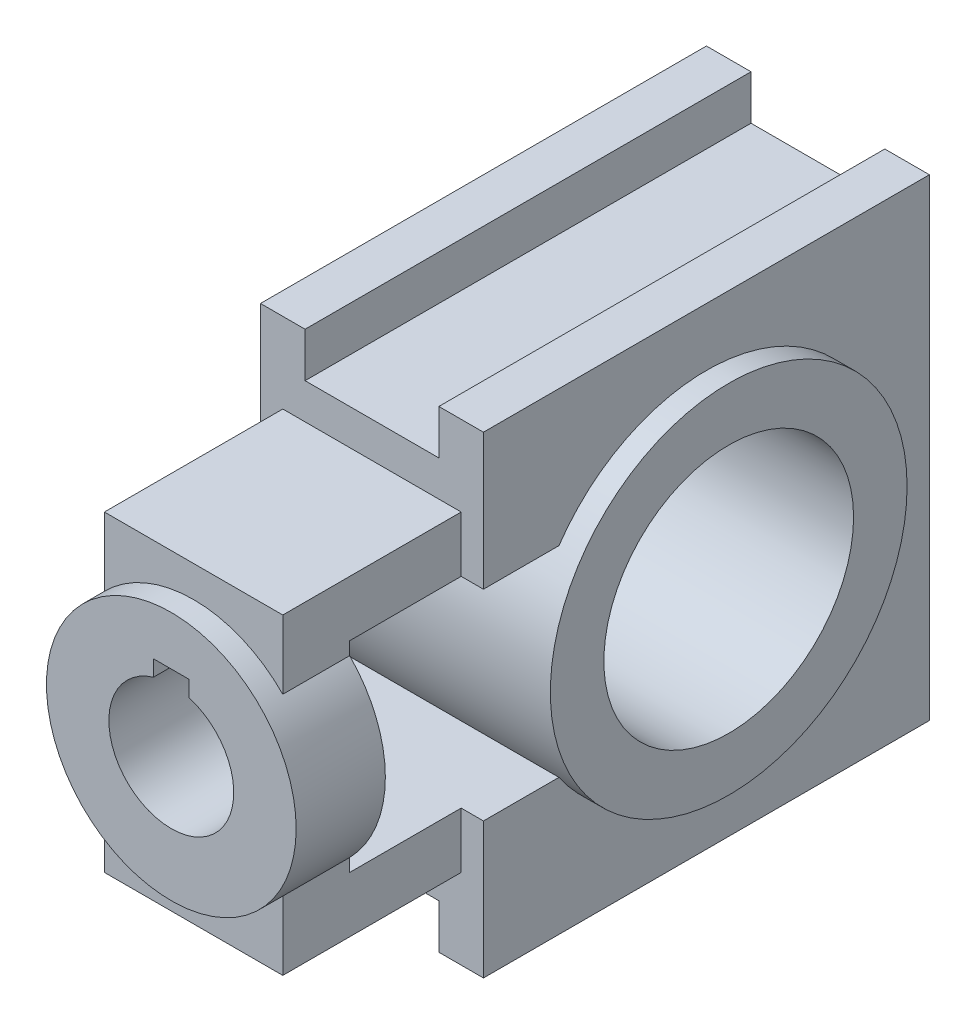
ISO-10303-21;
HEADER;
FILE_DESCRIPTION(('STEP AP214'),'2;1');
FILE_NAME('part.step','',(''),(''),'','','');
FILE_SCHEMA(('AUTOMOTIVE_DESIGN { 1 0 10303 214 1 1 1 1 }'));
ENDSEC;
DATA;
#1=APPLICATION_CONTEXT('core data for automotive mechanical design processes');
#2=APPLICATION_PROTOCOL_DEFINITION('international standard','automotive_design',2000,#1);
#3=PRODUCT_CONTEXT('',#1,'mechanical');
#4=PRODUCT('Part','Part','',(#3));
#5=PRODUCT_RELATED_PRODUCT_CATEGORY('part','',(#4));
#6=PRODUCT_DEFINITION_FORMATION('','',#4);
#7=PRODUCT_DEFINITION_CONTEXT('part definition',#1,'design');
#8=PRODUCT_DEFINITION('design','',#6,#7);
#9=PRODUCT_DEFINITION_SHAPE('','',#8);
#10=(LENGTH_UNIT() NAMED_UNIT(*) SI_UNIT(.MILLI.,.METRE.));
#11=(NAMED_UNIT(*) PLANE_ANGLE_UNIT() SI_UNIT($,.RADIAN.));
#12=(NAMED_UNIT(*) SI_UNIT($,.STERADIAN.) SOLID_ANGLE_UNIT());
#13=UNCERTAINTY_MEASURE_WITH_UNIT(LENGTH_MEASURE(1.E-05),#10,'distance_accuracy_value','');
#14=(GEOMETRIC_REPRESENTATION_CONTEXT(3) GLOBAL_UNCERTAINTY_ASSIGNED_CONTEXT((#13)) GLOBAL_UNIT_ASSIGNED_CONTEXT((#10,
#11,#12)) REPRESENTATION_CONTEXT('',''));
#15=CARTESIAN_POINT('',(0.,0.,0.));
#16=DIRECTION('',(0.,0.,1.));
#17=DIRECTION('',(1.,0.,0.));
#18=AXIS2_PLACEMENT_3D('',#15,#16,#17);
#19=CARTESIAN_POINT('',(-50.,-53.,50.));
#20=DIRECTION('',(0.,-1.,0.));
#21=DIRECTION('',(0.,0.,-1.));
#22=AXIS2_PLACEMENT_3D('',#19,#20,#21);
#23=PLANE('',#22);
#24=DIRECTION('',(0.,0.,1.));
#25=VECTOR('',#24,1.);
#26=CARTESIAN_POINT('',(-10.,-53.,-50.));
#27=LINE('',#26,#25);
#28=CARTESIAN_POINT('',(-10.,-53.,-50.));
#29=VERTEX_POINT('',#28);
#30=CARTESIAN_POINT('',(-10.,-53.,50.));
#31=VERTEX_POINT('',#30);
#32=EDGE_CURVE('E261',#29,#31,#27,.T.);
#33=ORIENTED_EDGE('',*,*,#32,.F.);
#34=DIRECTION('',(1.,0.,0.));
#35=VECTOR('',#34,1.);
#36=CARTESIAN_POINT('',(-50.,-53.,-50.));
#37=LINE('',#36,#35);
#38=CARTESIAN_POINT('',(0.,-53.,-50.));
#39=VERTEX_POINT('',#38);
#40=EDGE_CURVE('E475',#29,#39,#37,.T.);
#41=ORIENTED_EDGE('',*,*,#40,.T.);
#42=DIRECTION('',(0.,0.,-1.));
#43=VECTOR('',#42,1.);
#44=CARTESIAN_POINT('',(0.,-53.,50.));
#45=LINE('',#44,#43);
#46=CARTESIAN_POINT('',(0.,-53.,50.));
#47=VERTEX_POINT('',#46);
#48=EDGE_CURVE('E448',#47,#39,#45,.T.);
#49=ORIENTED_EDGE('',*,*,#48,.F.);
#50=DIRECTION('',(1.,0.,0.));
#51=VECTOR('',#50,1.);
#52=CARTESIAN_POINT('',(-50.,-53.,50.));
#53=LINE('',#52,#51);
#54=EDGE_CURVE('E479',#31,#47,#53,.T.);
#55=ORIENTED_EDGE('',*,*,#54,.F.);
#56=EDGE_LOOP('',(#33,#41,#49,#55));
#57=FACE_BOUND('',#56,.T.);
#58=ADVANCED_FACE('F39',(#57),#23,.T.);
#59=CARTESIAN_POINT('',(-50.,0.,0.));
#60=DIRECTION('',(1.,0.,0.));
#61=DIRECTION('',(0.,0.,-1.));
#62=AXIS2_PLACEMENT_3D('',#59,#60,#61);
#63=PLANE('',#62);
#64=CARTESIAN_POINT('',(-50.,0.,0.));
#65=DIRECTION('',(-1.,0.,0.));
#66=DIRECTION('',(0.,0.,1.));
#67=AXIS2_PLACEMENT_3D('',#64,#65,#66);
#68=CIRCLE('',#67,40.);
#69=CARTESIAN_POINT('',(-50.,22.5,33.0718913883074));
#70=VERTEX_POINT('',#69);
#71=CARTESIAN_POINT('',(-50.,-22.5,33.0718913883074));
#72=VERTEX_POINT('',#71);
#73=EDGE_CURVE('E279',#70,#72,#68,.T.);
#74=ORIENTED_EDGE('',*,*,#73,.F.);
#75=DIRECTION('',(0.,0.,1.));
#76=VECTOR('',#75,1.);
#77=CARTESIAN_POINT('',(-50.,22.5,50.));
#78=LINE('',#77,#76);
#79=CARTESIAN_POINT('',(-50.,22.5,50.));
#80=VERTEX_POINT('',#79);
#81=EDGE_CURVE('E424',#70,#80,#78,.T.);
#82=ORIENTED_EDGE('',*,*,#81,.T.);
#83=DIRECTION('',(0.,-1.,0.));
#84=VECTOR('',#83,1.);
#85=CARTESIAN_POINT('',(-50.,53.,50.));
#86=LINE('',#85,#84);
#87=CARTESIAN_POINT('',(-50.,53.,50.));
#88=VERTEX_POINT('',#87);
#89=EDGE_CURVE('E455',#88,#80,#86,.T.);
#90=ORIENTED_EDGE('',*,*,#89,.F.);
#91=DIRECTION('',(0.,0.,1.));
#92=VECTOR('',#91,1.);
#93=CARTESIAN_POINT('',(-50.,53.,-50.));
#94=LINE('',#93,#92);
#95=CARTESIAN_POINT('',(-50.,53.,-50.));
#96=VERTEX_POINT('',#95);
#97=EDGE_CURVE('E446',#96,#88,#94,.T.);
#98=ORIENTED_EDGE('',*,*,#97,.F.);
#99=DIRECTION('',(0.,1.,0.));
#100=VECTOR('',#99,1.);
#101=CARTESIAN_POINT('',(-50.,-53.,-50.));
#102=LINE('',#101,#100);
#103=CARTESIAN_POINT('',(-50.,-53.,-50.));
#104=VERTEX_POINT('',#103);
#105=EDGE_CURVE('E450',#104,#96,#102,.T.);
#106=ORIENTED_EDGE('',*,*,#105,.F.);
#107=DIRECTION('',(0.,0.,-1.));
#108=VECTOR('',#107,1.);
#109=CARTESIAN_POINT('',(-50.,-53.,50.));
#110=LINE('',#109,#108);
#111=CARTESIAN_POINT('',(-50.,-53.,50.));
#112=VERTEX_POINT('',#111);
#113=EDGE_CURVE('E456',#112,#104,#110,.T.);
#114=ORIENTED_EDGE('',*,*,#113,.F.);
#115=CARTESIAN_POINT('',(-50.,-22.5,50.));
#116=VERTEX_POINT('',#115);
#117=EDGE_CURVE('E452',#116,#112,#86,.T.);
#118=ORIENTED_EDGE('',*,*,#117,.F.);
#119=DIRECTION('',(0.,0.,-1.));
#120=VECTOR('',#119,1.);
#121=CARTESIAN_POINT('',(-50.,-22.5,50.));
#122=LINE('',#121,#120);
#123=EDGE_CURVE('E422',#116,#72,#122,.T.);
#124=ORIENTED_EDGE('',*,*,#123,.T.);
#125=EDGE_LOOP('',(#74,#82,#90,#98,#106,#114,#118,#124));
#126=FACE_BOUND('',#125,.T.);
#127=ADVANCED_FACE('F539',(#126),#63,.F.);
#128=CARTESIAN_POINT('',(-45.,0.,90.));
#129=DIRECTION('',(0.,0.,1.));
#130=DIRECTION('',(1.,0.,0.));
#131=AXIS2_PLACEMENT_3D('',#128,#129,#130);
#132=PLANE('',#131);
#133=CARTESIAN_POINT('',(-25.,0.,90.));
#134=DIRECTION('',(0.,0.,1.));
#135=DIRECTION('',(1.,0.,0.));
#136=AXIS2_PLACEMENT_3D('',#133,#134,#135);
#137=CIRCLE('',#136,28.);
#138=CARTESIAN_POINT('',(-5.,19.5959179422654,90.));
#139=VERTEX_POINT('',#138);
#140=CARTESIAN_POINT('',(-45.,19.5959179422654,90.));
#141=VERTEX_POINT('',#140);
#142=EDGE_CURVE('E314',#139,#141,#137,.T.);
#143=ORIENTED_EDGE('',*,*,#142,.F.);
#144=DIRECTION('',(0.,-1.,0.));
#145=VECTOR('',#144,1.);
#146=CARTESIAN_POINT('',(-5.,0.,90.));
#147=LINE('',#146,#145);
#148=CARTESIAN_POINT('',(-5.,35.,90.));
#149=VERTEX_POINT('',#148);
#150=EDGE_CURVE('E370',#149,#139,#147,.T.);
#151=ORIENTED_EDGE('',*,*,#150,.F.);
#152=DIRECTION('',(1.,0.,0.));
#153=VECTOR('',#152,1.);
#154=CARTESIAN_POINT('',(-45.,35.,90.));
#155=LINE('',#154,#153);
#156=CARTESIAN_POINT('',(-45.,35.,90.));
#157=VERTEX_POINT('',#156);
#158=EDGE_CURVE('E379',#157,#149,#155,.T.);
#159=ORIENTED_EDGE('',*,*,#158,.F.);
#160=DIRECTION('',(0.,-1.,0.));
#161=VECTOR('',#160,1.);
#162=CARTESIAN_POINT('',(-45.,0.,90.));
#163=LINE('',#162,#161);
#164=EDGE_CURVE('E344',#157,#141,#163,.T.);
#165=ORIENTED_EDGE('',*,*,#164,.T.);
#166=EDGE_LOOP('',(#143,#151,#159,#165));
#167=FACE_BOUND('',#166,.T.);
#168=ADVANCED_FACE('F560',(#167),#132,.T.);
#169=CARTESIAN_POINT('',(-45.,0.,0.));
#170=DIRECTION('',(1.,0.,0.));
#171=DIRECTION('',(0.,0.,-1.));
#172=AXIS2_PLACEMENT_3D('',#169,#170,#171);
#173=PLANE('',#172);
#174=DIRECTION('',(0.,1.,0.));
#175=VECTOR('',#174,1.);
#176=CARTESIAN_POINT('',(-45.,22.5,75.));
#177=LINE('',#176,#175);
#178=CARTESIAN_POINT('',(-45.,19.5959179422654,75.));
#179=VERTEX_POINT('',#178);
#180=CARTESIAN_POINT('',(-45.,22.5,75.));
#181=VERTEX_POINT('',#180);
#182=EDGE_CURVE('E330',#179,#181,#177,.T.);
#183=ORIENTED_EDGE('',*,*,#182,.F.);
#184=DIRECTION('',(0.,0.,1.));
#185=VECTOR('',#184,1.);
#186=CARTESIAN_POINT('',(-45.,19.5959179422654,75.));
#187=LINE('',#186,#185);
#188=EDGE_CURVE('E323',#179,#141,#187,.T.);
#189=ORIENTED_EDGE('',*,*,#188,.T.);
#190=ORIENTED_EDGE('',*,*,#164,.F.);
#191=DIRECTION('',(0.,0.,1.));
#192=VECTOR('',#191,1.);
#193=CARTESIAN_POINT('',(-45.,35.,90.));
#194=LINE('',#193,#192);
#195=CARTESIAN_POINT('',(-45.,35.,50.));
#196=VERTEX_POINT('',#195);
#197=EDGE_CURVE('E336',#196,#157,#194,.T.);
#198=ORIENTED_EDGE('',*,*,#197,.F.);
#199=DIRECTION('',(0.,1.,0.));
#200=VECTOR('',#199,1.);
#201=CARTESIAN_POINT('',(-45.,35.,50.));
#202=LINE('',#201,#200);
#203=CARTESIAN_POINT('',(-45.,22.5,50.));
#204=VERTEX_POINT('',#203);
#205=EDGE_CURVE('E337',#204,#196,#202,.T.);
#206=ORIENTED_EDGE('',*,*,#205,.F.);
#207=DIRECTION('',(0.,0.,-1.));
#208=VECTOR('',#207,1.);
#209=CARTESIAN_POINT('',(-45.,22.5,50.));
#210=LINE('',#209,#208);
#211=EDGE_CURVE('E333',#181,#204,#210,.T.);
#212=ORIENTED_EDGE('',*,*,#211,.F.);
#213=EDGE_LOOP('',(#183,#189,#190,#198,#206,#212));
#214=FACE_BOUND('',#213,.T.);
#215=ADVANCED_FACE('F550',(#214),#173,.F.);
#216=CARTESIAN_POINT('',(-5.,0.,0.));
#217=DIRECTION('',(1.,0.,0.));
#218=DIRECTION('',(0.,0.,-1.));
#219=AXIS2_PLACEMENT_3D('',#216,#217,#218);
#220=PLANE('',#219);
#221=DIRECTION('',(0.,0.,1.));
#222=VECTOR('',#221,1.);
#223=CARTESIAN_POINT('',(-5.,19.5959179422654,75.));
#224=LINE('',#223,#222);
#225=CARTESIAN_POINT('',(-5.,19.5959179422654,75.));
#226=VERTEX_POINT('',#225);
#227=EDGE_CURVE('E11',#226,#139,#224,.T.);
#228=ORIENTED_EDGE('',*,*,#227,.F.);
#229=DIRECTION('',(0.,1.,0.));
#230=VECTOR('',#229,1.);
#231=CARTESIAN_POINT('',(-5.,22.5,75.));
#232=LINE('',#231,#230);
#233=CARTESIAN_POINT('',(-5.,22.5,75.));
#234=VERTEX_POINT('',#233);
#235=EDGE_CURVE('E353',#226,#234,#232,.T.);
#236=ORIENTED_EDGE('',*,*,#235,.T.);
#237=DIRECTION('',(0.,0.,-1.));
#238=VECTOR('',#237,1.);
#239=CARTESIAN_POINT('',(-5.,22.5,50.));
#240=LINE('',#239,#238);
#241=CARTESIAN_POINT('',(-5.,22.5,50.));
#242=VERTEX_POINT('',#241);
#243=EDGE_CURVE('E357',#234,#242,#240,.T.);
#244=ORIENTED_EDGE('',*,*,#243,.T.);
#245=DIRECTION('',(0.,1.,0.));
#246=VECTOR('',#245,1.);
#247=CARTESIAN_POINT('',(-5.,35.,50.));
#248=LINE('',#247,#246);
#249=CARTESIAN_POINT('',(-5.,35.,50.));
#250=VERTEX_POINT('',#249);
#251=EDGE_CURVE('E359',#242,#250,#248,.T.);
#252=ORIENTED_EDGE('',*,*,#251,.T.);
#253=DIRECTION('',(0.,0.,1.));
#254=VECTOR('',#253,1.);
#255=CARTESIAN_POINT('',(-5.,35.,90.));
#256=LINE('',#255,#254);
#257=EDGE_CURVE('E361',#250,#149,#256,.T.);
#258=ORIENTED_EDGE('',*,*,#257,.T.);
#259=ORIENTED_EDGE('',*,*,#150,.T.);
#260=EDGE_LOOP('',(#228,#236,#244,#252,#258,#259));
#261=FACE_BOUND('',#260,.T.);
#262=ADVANCED_FACE('F551',(#261),#220,.T.);
#263=CARTESIAN_POINT('',(-50.,53.,50.));
#264=DIRECTION('',(0.,0.,1.));
#265=DIRECTION('',(0.,-1.,0.));
#266=AXIS2_PLACEMENT_3D('',#263,#264,#265);
#267=PLANE('',#266);
#268=DIRECTION('',(1.,0.,0.));
#269=VECTOR('',#268,1.);
#270=CARTESIAN_POINT('',(-50.,22.5,50.));
#271=LINE('',#270,#269);
#272=EDGE_CURVE('E432',#80,#204,#271,.T.);
#273=ORIENTED_EDGE('',*,*,#272,.T.);
#274=ORIENTED_EDGE('',*,*,#205,.T.);
#275=DIRECTION('',(1.,0.,0.));
#276=VECTOR('',#275,1.);
#277=CARTESIAN_POINT('',(-45.,35.,50.));
#278=LINE('',#277,#276);
#279=EDGE_CURVE('E384',#196,#250,#278,.T.);
#280=ORIENTED_EDGE('',*,*,#279,.T.);
#281=ORIENTED_EDGE('',*,*,#251,.F.);
#282=CARTESIAN_POINT('',(0.,22.5,50.));
#283=VERTEX_POINT('',#282);
#284=EDGE_CURVE('E440',#242,#283,#271,.T.);
#285=ORIENTED_EDGE('',*,*,#284,.T.);
#286=DIRECTION('',(0.,-1.,0.));
#287=VECTOR('',#286,1.);
#288=CARTESIAN_POINT('',(0.,53.,50.));
#289=LINE('',#288,#287);
#290=CARTESIAN_POINT('',(0.,53.,50.));
#291=VERTEX_POINT('',#290);
#292=EDGE_CURVE('E470',#291,#283,#289,.T.);
#293=ORIENTED_EDGE('',*,*,#292,.F.);
#294=DIRECTION('',(1.,0.,0.));
#295=VECTOR('',#294,1.);
#296=CARTESIAN_POINT('',(-50.,53.,50.));
#297=LINE('',#296,#295);
#298=CARTESIAN_POINT('',(-10.,53.,50.));
#299=VERTEX_POINT('',#298);
#300=EDGE_CURVE('E477',#299,#291,#297,.T.);
#301=ORIENTED_EDGE('',*,*,#300,.F.);
#302=DIRECTION('',(0.,1.,0.));
#303=VECTOR('',#302,1.);
#304=CARTESIAN_POINT('',(-10.,43.,50.));
#305=LINE('',#304,#303);
#306=CARTESIAN_POINT('',(-10.,43.,50.));
#307=VERTEX_POINT('',#306);
#308=EDGE_CURVE('E408',#307,#299,#305,.T.);
#309=ORIENTED_EDGE('',*,*,#308,.F.);
#310=DIRECTION('',(1.,0.,0.));
#311=VECTOR('',#310,1.);
#312=CARTESIAN_POINT('',(-40.,43.,50.));
#313=LINE('',#312,#311);
#314=CARTESIAN_POINT('',(-40.,43.,50.));
#315=VERTEX_POINT('',#314);
#316=EDGE_CURVE('E392',#315,#307,#313,.T.);
#317=ORIENTED_EDGE('',*,*,#316,.F.);
#318=DIRECTION('',(0.,1.,0.));
#319=VECTOR('',#318,1.);
#320=CARTESIAN_POINT('',(-40.,43.,50.));
#321=LINE('',#320,#319);
#322=CARTESIAN_POINT('',(-40.,53.,50.));
#323=VERTEX_POINT('',#322);
#324=EDGE_CURVE('E407',#315,#323,#321,.T.);
#325=ORIENTED_EDGE('',*,*,#324,.T.);
#326=EDGE_CURVE('E476',#88,#323,#297,.T.);
#327=ORIENTED_EDGE('',*,*,#326,.F.);
#328=ORIENTED_EDGE('',*,*,#89,.T.);
#329=EDGE_LOOP('',(#273,#274,#280,#281,#285,#293,#301,#309,#317,#325,#327,#328));
#330=FACE_BOUND('',#329,.T.);
#331=ADVANCED_FACE('F522',(#330),#267,.T.);
#332=DIRECTION('',(0.,-1.,0.));
#333=VECTOR('',#332,1.);
#334=CARTESIAN_POINT('',(-10.,-43.,50.));
#335=LINE('',#334,#333);
#336=CARTESIAN_POINT('',(-10.,-43.,50.));
#337=VERTEX_POINT('',#336);
#338=EDGE_CURVE('E277',#337,#31,#335,.T.);
#339=ORIENTED_EDGE('',*,*,#338,.T.);
#340=ORIENTED_EDGE('',*,*,#54,.T.);
#341=CARTESIAN_POINT('',(0.,-22.5,50.));
#342=VERTEX_POINT('',#341);
#343=EDGE_CURVE('E467',#342,#47,#289,.T.);
#344=ORIENTED_EDGE('',*,*,#343,.F.);
#345=DIRECTION('',(1.,0.,0.));
#346=VECTOR('',#345,1.);
#347=CARTESIAN_POINT('',(-50.,-22.5,50.));
#348=LINE('',#347,#346);
#349=CARTESIAN_POINT('',(-5.,-22.5,50.));
#350=VERTEX_POINT('',#349);
#351=EDGE_CURVE('E429',#350,#342,#348,.T.);
#352=ORIENTED_EDGE('',*,*,#351,.F.);
#353=DIRECTION('',(0.,1.,0.));
#354=VECTOR('',#353,1.);
#355=CARTESIAN_POINT('',(-5.,-35.,50.));
#356=LINE('',#355,#354);
#357=CARTESIAN_POINT('',(-5.,-35.,50.));
#358=VERTEX_POINT('',#357);
#359=EDGE_CURVE('E328',#358,#350,#356,.T.);
#360=ORIENTED_EDGE('',*,*,#359,.F.);
#361=DIRECTION('',(1.,0.,0.));
#362=VECTOR('',#361,1.);
#363=CARTESIAN_POINT('',(-45.,-35.,50.));
#364=LINE('',#363,#362);
#365=CARTESIAN_POINT('',(-45.,-35.,50.));
#366=VERTEX_POINT('',#365);
#367=EDGE_CURVE('E372',#366,#358,#364,.T.);
#368=ORIENTED_EDGE('',*,*,#367,.F.);
#369=DIRECTION('',(0.,1.,0.));
#370=VECTOR('',#369,1.);
#371=CARTESIAN_POINT('',(-45.,-35.,50.));
#372=LINE('',#371,#370);
#373=CARTESIAN_POINT('',(-45.,-22.5,50.));
#374=VERTEX_POINT('',#373);
#375=EDGE_CURVE('E346',#366,#374,#372,.T.);
#376=ORIENTED_EDGE('',*,*,#375,.T.);
#377=EDGE_CURVE('E443',#116,#374,#348,.T.);
#378=ORIENTED_EDGE('',*,*,#377,.F.);
#379=ORIENTED_EDGE('',*,*,#117,.T.);
#380=CARTESIAN_POINT('',(-40.,-53.,50.));
#381=VERTEX_POINT('',#380);
#382=EDGE_CURVE('E270',#112,#381,#53,.T.);
#383=ORIENTED_EDGE('',*,*,#382,.T.);
#384=DIRECTION('',(0.,-1.,0.));
#385=VECTOR('',#384,1.);
#386=CARTESIAN_POINT('',(-40.,-43.,50.));
#387=LINE('',#386,#385);
#388=CARTESIAN_POINT('',(-40.,-43.,50.));
#389=VERTEX_POINT('',#388);
#390=EDGE_CURVE('E250',#389,#381,#387,.T.);
#391=ORIENTED_EDGE('',*,*,#390,.F.);
#392=DIRECTION('',(-1.,0.,0.));
#393=VECTOR('',#392,1.);
#394=CARTESIAN_POINT('',(-10.,-43.,50.));
#395=LINE('',#394,#393);
#396=EDGE_CURVE('E254',#337,#389,#395,.T.);
#397=ORIENTED_EDGE('',*,*,#396,.F.);
#398=EDGE_LOOP('',(#339,#340,#344,#352,#360,#368,#376,#378,#379,#383,#391,#397));
#399=FACE_BOUND('',#398,.T.);
#400=ADVANCED_FACE('F262',(#399),#267,.T.);
#401=CARTESIAN_POINT('',(-50.,53.,-50.));
#402=DIRECTION('',(0.,1.,0.));
#403=DIRECTION('',(0.,0.,1.));
#404=AXIS2_PLACEMENT_3D('',#401,#402,#403);
#405=PLANE('',#404);
#406=DIRECTION('',(0.,0.,-1.));
#407=VECTOR('',#406,1.);
#408=CARTESIAN_POINT('',(-10.,53.,50.));
#409=LINE('',#408,#407);
#410=CARTESIAN_POINT('',(-10.,53.,-50.));
#411=VERTEX_POINT('',#410);
#412=EDGE_CURVE('E391',#299,#411,#409,.T.);
#413=ORIENTED_EDGE('',*,*,#412,.F.);
#414=ORIENTED_EDGE('',*,*,#300,.T.);
#415=DIRECTION('',(0.,0.,1.));
#416=VECTOR('',#415,1.);
#417=CARTESIAN_POINT('',(0.,53.,-50.));
#418=LINE('',#417,#416);
#419=CARTESIAN_POINT('',(0.,53.,-50.));
#420=VERTEX_POINT('',#419);
#421=EDGE_CURVE('E463',#420,#291,#418,.T.);
#422=ORIENTED_EDGE('',*,*,#421,.F.);
#423=DIRECTION('',(1.,0.,0.));
#424=VECTOR('',#423,1.);
#425=CARTESIAN_POINT('',(-50.,53.,-50.));
#426=LINE('',#425,#424);
#427=EDGE_CURVE('E457',#411,#420,#426,.T.);
#428=ORIENTED_EDGE('',*,*,#427,.F.);
#429=EDGE_LOOP('',(#413,#414,#422,#428));
#430=FACE_BOUND('',#429,.T.);
#431=ADVANCED_FACE('F524',(#430),#405,.T.);
#432=DIRECTION('',(0.,0.,-1.));
#433=VECTOR('',#432,1.);
#434=CARTESIAN_POINT('',(-40.,-53.,50.));
#435=LINE('',#434,#433);
#436=CARTESIAN_POINT('',(-40.,-53.,-50.));
#437=VERTEX_POINT('',#436);
#438=EDGE_CURVE('E595',#381,#437,#435,.T.);
#439=ORIENTED_EDGE('',*,*,#438,.F.);
#440=ORIENTED_EDGE('',*,*,#382,.F.);
#441=ORIENTED_EDGE('',*,*,#113,.T.);
#442=EDGE_CURVE('E423',#104,#437,#37,.T.);
#443=ORIENTED_EDGE('',*,*,#442,.T.);
#444=EDGE_LOOP('',(#439,#440,#441,#443));
#445=FACE_BOUND('',#444,.T.);
#446=ADVANCED_FACE('F577',(#445),#23,.T.);
#447=DIRECTION('',(0.,0.,1.));
#448=VECTOR('',#447,1.);
#449=CARTESIAN_POINT('',(-40.,53.,-50.));
#450=LINE('',#449,#448);
#451=CARTESIAN_POINT('',(-40.,53.,-50.));
#452=VERTEX_POINT('',#451);
#453=EDGE_CURVE('E376',#452,#323,#450,.T.);
#454=ORIENTED_EDGE('',*,*,#453,.F.);
#455=EDGE_CURVE('E482',#96,#452,#426,.T.);
#456=ORIENTED_EDGE('',*,*,#455,.F.);
#457=ORIENTED_EDGE('',*,*,#97,.T.);
#458=ORIENTED_EDGE('',*,*,#326,.T.);
#459=EDGE_LOOP('',(#454,#456,#457,#458));
#460=FACE_BOUND('',#459,.T.);
#461=ADVANCED_FACE('F585',(#460),#405,.T.);
#462=CARTESIAN_POINT('',(-50.,0.,-50.));
#463=DIRECTION('',(0.,0.,-1.));
#464=DIRECTION('',(-1.,0.,0.));
#465=AXIS2_PLACEMENT_3D('',#462,#463,#464);
#466=PLANE('',#465);
#467=DIRECTION('',(0.,-1.,0.));
#468=VECTOR('',#467,1.);
#469=CARTESIAN_POINT('',(-10.,-43.,-50.));
#470=LINE('',#469,#468);
#471=CARTESIAN_POINT('',(-10.,-43.,-50.));
#472=VERTEX_POINT('',#471);
#473=EDGE_CURVE('E269',#472,#29,#470,.T.);
#474=ORIENTED_EDGE('',*,*,#473,.F.);
#475=DIRECTION('',(1.,0.,0.));
#476=VECTOR('',#475,1.);
#477=CARTESIAN_POINT('',(-40.,-43.,-50.));
#478=LINE('',#477,#476);
#479=CARTESIAN_POINT('',(-40.,-43.,-50.));
#480=VERTEX_POINT('',#479);
#481=EDGE_CURVE('E255',#480,#472,#478,.T.);
#482=ORIENTED_EDGE('',*,*,#481,.F.);
#483=DIRECTION('',(0.,-1.,0.));
#484=VECTOR('',#483,1.);
#485=CARTESIAN_POINT('',(-40.,-43.,-50.));
#486=LINE('',#485,#484);
#487=EDGE_CURVE('E249',#480,#437,#486,.T.);
#488=ORIENTED_EDGE('',*,*,#487,.T.);
#489=ORIENTED_EDGE('',*,*,#442,.F.);
#490=ORIENTED_EDGE('',*,*,#105,.T.);
#491=ORIENTED_EDGE('',*,*,#455,.T.);
#492=DIRECTION('',(0.,1.,0.));
#493=VECTOR('',#492,1.);
#494=CARTESIAN_POINT('',(-40.,43.,-50.));
#495=LINE('',#494,#493);
#496=CARTESIAN_POINT('',(-40.,43.,-50.));
#497=VERTEX_POINT('',#496);
#498=EDGE_CURVE('E399',#497,#452,#495,.T.);
#499=ORIENTED_EDGE('',*,*,#498,.F.);
#500=DIRECTION('',(-1.,0.,0.));
#501=VECTOR('',#500,1.);
#502=CARTESIAN_POINT('',(-10.,43.,-50.));
#503=LINE('',#502,#501);
#504=CARTESIAN_POINT('',(-10.,43.,-50.));
#505=VERTEX_POINT('',#504);
#506=EDGE_CURVE('E387',#505,#497,#503,.T.);
#507=ORIENTED_EDGE('',*,*,#506,.F.);
#508=DIRECTION('',(0.,1.,0.));
#509=VECTOR('',#508,1.);
#510=CARTESIAN_POINT('',(-10.,43.,-50.));
#511=LINE('',#510,#509);
#512=EDGE_CURVE('E405',#505,#411,#511,.T.);
#513=ORIENTED_EDGE('',*,*,#512,.T.);
#514=ORIENTED_EDGE('',*,*,#427,.T.);
#515=DIRECTION('',(0.,1.,0.));
#516=VECTOR('',#515,1.);
#517=CARTESIAN_POINT('',(0.,0.,-50.));
#518=LINE('',#517,#516);
#519=EDGE_CURVE('E436',#39,#420,#518,.T.);
#520=ORIENTED_EDGE('',*,*,#519,.F.);
#521=ORIENTED_EDGE('',*,*,#40,.F.);
#522=EDGE_LOOP('',(#474,#482,#488,#489,#490,#491,#499,#507,#513,#514,#520,#521));
#523=FACE_BOUND('',#522,.T.);
#524=ADVANCED_FACE('F41',(#523),#466,.T.);
#525=CARTESIAN_POINT('',(0.,0.,0.));
#526=DIRECTION('',(1.,0.,0.));
#527=DIRECTION('',(0.,0.,-1.));
#528=AXIS2_PLACEMENT_3D('',#525,#526,#527);
#529=PLANE('',#528);
#530=CARTESIAN_POINT('',(0.,0.,0.));
#531=DIRECTION('',(1.,0.,0.));
#532=DIRECTION('',(0.,0.,-1.));
#533=AXIS2_PLACEMENT_3D('',#530,#531,#532);
#534=CIRCLE('',#533,40.);
#535=CARTESIAN_POINT('',(0.,-22.5,33.0718913883074));
#536=VERTEX_POINT('',#535);
#537=CARTESIAN_POINT('',(0.,22.5,33.0718913883074));
#538=VERTEX_POINT('',#537);
#539=EDGE_CURVE('E418',#536,#538,#534,.T.);
#540=ORIENTED_EDGE('',*,*,#539,.F.);
#541=DIRECTION('',(0.,0.,-1.));
#542=VECTOR('',#541,1.);
#543=CARTESIAN_POINT('',(0.,-22.5,50.));
#544=LINE('',#543,#542);
#545=EDGE_CURVE('E420',#342,#536,#544,.T.);
#546=ORIENTED_EDGE('',*,*,#545,.F.);
#547=ORIENTED_EDGE('',*,*,#343,.T.);
#548=ORIENTED_EDGE('',*,*,#48,.T.);
#549=ORIENTED_EDGE('',*,*,#519,.T.);
#550=ORIENTED_EDGE('',*,*,#421,.T.);
#551=ORIENTED_EDGE('',*,*,#292,.T.);
#552=DIRECTION('',(0.,0.,1.));
#553=VECTOR('',#552,1.);
#554=CARTESIAN_POINT('',(0.,22.5,50.));
#555=LINE('',#554,#553);
#556=EDGE_CURVE('E428',#538,#283,#555,.T.);
#557=ORIENTED_EDGE('',*,*,#556,.F.);
#558=EDGE_LOOP('',(#540,#546,#547,#548,#549,#550,#551,#557));
#559=FACE_BOUND('',#558,.T.);
#560=ADVANCED_FACE('F508',(#559),#529,.T.);
#561=CARTESIAN_POINT('',(-50.,22.5,50.));
#562=DIRECTION('',(0.,1.,0.));
#563=DIRECTION('',(0.,0.,1.));
#564=AXIS2_PLACEMENT_3D('',#561,#562,#563);
#565=PLANE('',#564);
#566=ORIENTED_EDGE('',*,*,#556,.T.);
#567=ORIENTED_EDGE('',*,*,#284,.F.);
#568=ORIENTED_EDGE('',*,*,#243,.F.);
#569=DIRECTION('',(1.,0.,0.));
#570=VECTOR('',#569,1.);
#571=CARTESIAN_POINT('',(-45.,22.5,75.));
#572=LINE('',#571,#570);
#573=EDGE_CURVE('E383',#181,#234,#572,.T.);
#574=ORIENTED_EDGE('',*,*,#573,.F.);
#575=ORIENTED_EDGE('',*,*,#211,.T.);
#576=ORIENTED_EDGE('',*,*,#272,.F.);
#577=ORIENTED_EDGE('',*,*,#81,.F.);
#578=DIRECTION('',(1.,0.,0.));
#579=VECTOR('',#578,1.);
#580=CARTESIAN_POINT('',(-50.,22.5,33.0718913883074));
#581=LINE('',#580,#579);
#582=EDGE_CURVE('E438',#70,#538,#581,.T.);
#583=ORIENTED_EDGE('',*,*,#582,.T.);
#584=EDGE_LOOP('',(#566,#567,#568,#574,#575,#576,#577,#583));
#585=FACE_BOUND('',#584,.T.);
#586=ADVANCED_FACE('F529',(#585),#565,.F.);
#587=CARTESIAN_POINT('',(-50.,-22.5,50.));
#588=DIRECTION('',(0.,-1.,0.));
#589=DIRECTION('',(0.,0.,-1.));
#590=AXIS2_PLACEMENT_3D('',#587,#588,#589);
#591=PLANE('',#590);
#592=ORIENTED_EDGE('',*,*,#545,.T.);
#593=DIRECTION('',(1.,0.,0.));
#594=VECTOR('',#593,1.);
#595=CARTESIAN_POINT('',(-50.,-22.5,33.0718913883074));
#596=LINE('',#595,#594);
#597=EDGE_CURVE('E441',#72,#536,#596,.T.);
#598=ORIENTED_EDGE('',*,*,#597,.F.);
#599=ORIENTED_EDGE('',*,*,#123,.F.);
#600=ORIENTED_EDGE('',*,*,#377,.T.);
#601=DIRECTION('',(0.,0.,1.));
#602=VECTOR('',#601,1.);
#603=CARTESIAN_POINT('',(-45.,-22.5,75.));
#604=LINE('',#603,#602);
#605=CARTESIAN_POINT('',(-45.,-22.5,75.));
#606=VERTEX_POINT('',#605);
#607=EDGE_CURVE('E321',#374,#606,#604,.T.);
#608=ORIENTED_EDGE('',*,*,#607,.T.);
#609=DIRECTION('',(1.,0.,0.));
#610=VECTOR('',#609,1.);
#611=CARTESIAN_POINT('',(-45.,-22.5,75.));
#612=LINE('',#611,#610);
#613=CARTESIAN_POINT('',(-5.,-22.5,75.));
#614=VERTEX_POINT('',#613);
#615=EDGE_CURVE('E347',#606,#614,#612,.T.);
#616=ORIENTED_EDGE('',*,*,#615,.T.);
#617=DIRECTION('',(0.,0.,1.));
#618=VECTOR('',#617,1.);
#619=CARTESIAN_POINT('',(-5.,-22.5,75.));
#620=LINE('',#619,#618);
#621=EDGE_CURVE('E325',#350,#614,#620,.T.);
#622=ORIENTED_EDGE('',*,*,#621,.F.);
#623=ORIENTED_EDGE('',*,*,#351,.T.);
#624=EDGE_LOOP('',(#592,#598,#599,#600,#608,#616,#622,#623));
#625=FACE_BOUND('',#624,.T.);
#626=ADVANCED_FACE('F501',(#625),#591,.F.);
#627=CARTESIAN_POINT('',(-50.,0.,0.));
#628=DIRECTION('',(1.,0.,0.));
#629=DIRECTION('',(0.,0.,-1.));
#630=AXIS2_PLACEMENT_3D('',#627,#628,#629);
#631=CYLINDRICAL_SURFACE('',#630,40.);
#632=ORIENTED_EDGE('',*,*,#582,.F.);
#633=ORIENTED_EDGE('',*,*,#73,.T.);
#634=ORIENTED_EDGE('',*,*,#597,.T.);
#635=ORIENTED_EDGE('',*,*,#539,.T.);
#636=EDGE_LOOP('',(#632,#633,#634,#635));
#637=FACE_BOUND('',#636,.T.);
#638=CARTESIAN_POINT('',(5.,0.,0.));
#639=DIRECTION('',(1.,0.,0.));
#640=DIRECTION('',(0.,0.,-1.));
#641=AXIS2_PLACEMENT_3D('',#638,#639,#640);
#642=CIRCLE('',#641,40.);
#643=CARTESIAN_POINT('',(5.,0.,-40.));
#644=VERTEX_POINT('',#643);
#645=EDGE_CURVE('E413',#644,#644,#642,.T.);
#646=ORIENTED_EDGE('',*,*,#645,.F.);
#647=EDGE_LOOP('',(#646));
#648=FACE_BOUND('',#647,.T.);
#649=CARTESIAN_POINT('',(-55.,0.,0.));
#650=DIRECTION('',(-1.,0.,0.));
#651=DIRECTION('',(0.,0.,1.));
#652=AXIS2_PLACEMENT_3D('',#649,#650,#651);
#653=CIRCLE('',#652,40.);
#654=CARTESIAN_POINT('',(-55.,0.,40.));
#655=VERTEX_POINT('',#654);
#656=EDGE_CURVE('E280',#655,#655,#653,.T.);
#657=ORIENTED_EDGE('',*,*,#656,.F.);
#658=EDGE_LOOP('',(#657));
#659=FACE_BOUND('',#658,.T.);
#660=ADVANCED_FACE('F534',(#637,#648,#659),#631,.T.);
#661=CARTESIAN_POINT('',(5.,0.,0.));
#662=DIRECTION('',(1.,0.,0.));
#663=DIRECTION('',(0.,0.,-1.));
#664=AXIS2_PLACEMENT_3D('',#661,#662,#663);
#665=PLANE('',#664);
#666=CARTESIAN_POINT('',(5.,0.,0.));
#667=DIRECTION('',(1.,0.,0.));
#668=DIRECTION('',(0.,0.,-1.));
#669=AXIS2_PLACEMENT_3D('',#666,#667,#668);
#670=CIRCLE('',#669,28.);
#671=CARTESIAN_POINT('',(5.,0.,-28.));
#672=VERTEX_POINT('',#671);
#673=EDGE_CURVE('E403',#672,#672,#670,.T.);
#674=ORIENTED_EDGE('',*,*,#673,.F.);
#675=EDGE_LOOP('',(#674));
#676=FACE_BOUND('',#675,.T.);
#677=ORIENTED_EDGE('',*,*,#645,.T.);
#678=EDGE_LOOP('',(#677));
#679=FACE_BOUND('',#678,.T.);
#680=ADVANCED_FACE('F621',(#676,#679),#665,.T.);
#681=CARTESIAN_POINT('',(-108.,0.,0.));
#682=DIRECTION('',(1.,0.,0.));
#683=DIRECTION('',(0.,0.,-1.));
#684=AXIS2_PLACEMENT_3D('',#681,#682,#683);
#685=CYLINDRICAL_SURFACE('',#684,28.);
#686=ORIENTED_EDGE('',*,*,#673,.T.);
#687=EDGE_LOOP('',(#686));
#688=FACE_BOUND('',#687,.T.);
#689=CARTESIAN_POINT('',(-55.,0.,0.));
#690=DIRECTION('',(-1.,0.,0.));
#691=DIRECTION('',(0.,0.,1.));
#692=AXIS2_PLACEMENT_3D('',#689,#690,#691);
#693=CIRCLE('',#692,28.);
#694=CARTESIAN_POINT('',(-55.,0.,28.));
#695=VERTEX_POINT('',#694);
#696=EDGE_CURVE('E274',#695,#695,#693,.T.);
#697=ORIENTED_EDGE('',*,*,#696,.T.);
#698=EDGE_LOOP('',(#697));
#699=FACE_BOUND('',#698,.T.);
#700=ADVANCED_FACE('F618',(#688,#699),#685,.F.);
#701=CARTESIAN_POINT('',(-10.,43.,50.));
#702=DIRECTION('',(1.,0.,0.));
#703=DIRECTION('',(0.,0.,-1.));
#704=AXIS2_PLACEMENT_3D('',#701,#702,#703);
#705=PLANE('',#704);
#706=ORIENTED_EDGE('',*,*,#412,.T.);
#707=ORIENTED_EDGE('',*,*,#512,.F.);
#708=DIRECTION('',(0.,0.,-1.));
#709=VECTOR('',#708,1.);
#710=CARTESIAN_POINT('',(-10.,43.,50.));
#711=LINE('',#710,#709);
#712=EDGE_CURVE('E400',#307,#505,#711,.T.);
#713=ORIENTED_EDGE('',*,*,#712,.F.);
#714=ORIENTED_EDGE('',*,*,#308,.T.);
#715=EDGE_LOOP('',(#706,#707,#713,#714));
#716=FACE_BOUND('',#715,.T.);
#717=ADVANCED_FACE('F614',(#716),#705,.F.);
#718=CARTESIAN_POINT('',(-40.,43.,-50.));
#719=DIRECTION('',(-1.,0.,0.));
#720=DIRECTION('',(0.,0.,1.));
#721=AXIS2_PLACEMENT_3D('',#718,#719,#720);
#722=PLANE('',#721);
#723=ORIENTED_EDGE('',*,*,#453,.T.);
#724=ORIENTED_EDGE('',*,*,#324,.F.);
#725=DIRECTION('',(0.,0.,1.));
#726=VECTOR('',#725,1.);
#727=CARTESIAN_POINT('',(-40.,43.,-50.));
#728=LINE('',#727,#726);
#729=EDGE_CURVE('E394',#497,#315,#728,.T.);
#730=ORIENTED_EDGE('',*,*,#729,.F.);
#731=ORIENTED_EDGE('',*,*,#498,.T.);
#732=EDGE_LOOP('',(#723,#724,#730,#731));
#733=FACE_BOUND('',#732,.T.);
#734=ADVANCED_FACE('F606',(#733),#722,.F.);
#735=CARTESIAN_POINT('',(0.,43.,0.));
#736=DIRECTION('',(0.,1.,0.));
#737=DIRECTION('',(0.,0.,1.));
#738=AXIS2_PLACEMENT_3D('',#735,#736,#737);
#739=PLANE('',#738);
#740=ORIENTED_EDGE('',*,*,#506,.T.);
#741=ORIENTED_EDGE('',*,*,#729,.T.);
#742=ORIENTED_EDGE('',*,*,#316,.T.);
#743=ORIENTED_EDGE('',*,*,#712,.T.);
#744=EDGE_LOOP('',(#740,#741,#742,#743));
#745=FACE_BOUND('',#744,.T.);
#746=ADVANCED_FACE('F607',(#745),#739,.T.);
#747=CARTESIAN_POINT('',(-45.,-35.,90.));
#748=DIRECTION('',(0.,-1.,0.));
#749=DIRECTION('',(0.,0.,-1.));
#750=AXIS2_PLACEMENT_3D('',#747,#748,#749);
#751=PLANE('',#750);
#752=DIRECTION('',(0.,0.,-1.));
#753=VECTOR('',#752,1.);
#754=CARTESIAN_POINT('',(-5.,-35.,90.));
#755=LINE('',#754,#753);
#756=CARTESIAN_POINT('',(-5.,-35.,90.));
#757=VERTEX_POINT('',#756);
#758=EDGE_CURVE('E369',#757,#358,#755,.T.);
#759=ORIENTED_EDGE('',*,*,#758,.F.);
#760=DIRECTION('',(1.,0.,0.));
#761=VECTOR('',#760,1.);
#762=CARTESIAN_POINT('',(-45.,-35.,90.));
#763=LINE('',#762,#761);
#764=CARTESIAN_POINT('',(-45.,-35.,90.));
#765=VERTEX_POINT('',#764);
#766=EDGE_CURVE('E380',#765,#757,#763,.T.);
#767=ORIENTED_EDGE('',*,*,#766,.F.);
#768=DIRECTION('',(0.,0.,-1.));
#769=VECTOR('',#768,1.);
#770=CARTESIAN_POINT('',(-45.,-35.,90.));
#771=LINE('',#770,#769);
#772=EDGE_CURVE('E341',#765,#366,#771,.T.);
#773=ORIENTED_EDGE('',*,*,#772,.T.);
#774=ORIENTED_EDGE('',*,*,#367,.T.);
#775=EDGE_LOOP('',(#759,#767,#773,#774));
#776=FACE_BOUND('',#775,.T.);
#777=ADVANCED_FACE('F575',(#776),#751,.T.);
#778=CARTESIAN_POINT('',(-45.,-19.5959179422654,90.));
#779=VERTEX_POINT('',#778);
#780=CARTESIAN_POINT('',(-5.,-19.5959179422654,90.));
#781=VERTEX_POINT('',#780);
#782=EDGE_CURVE('E319',#779,#781,#137,.T.);
#783=ORIENTED_EDGE('',*,*,#782,.F.);
#784=EDGE_CURVE('E343',#779,#765,#163,.T.);
#785=ORIENTED_EDGE('',*,*,#784,.T.);
#786=ORIENTED_EDGE('',*,*,#766,.T.);
#787=EDGE_CURVE('E366',#781,#757,#147,.T.);
#788=ORIENTED_EDGE('',*,*,#787,.F.);
#789=EDGE_LOOP('',(#783,#785,#786,#788));
#790=FACE_BOUND('',#789,.T.);
#791=ADVANCED_FACE('F557',(#790),#132,.T.);
#792=CARTESIAN_POINT('',(-45.,35.,90.));
#793=DIRECTION('',(0.,1.,0.));
#794=DIRECTION('',(0.,0.,1.));
#795=AXIS2_PLACEMENT_3D('',#792,#793,#794);
#796=PLANE('',#795);
#797=ORIENTED_EDGE('',*,*,#257,.F.);
#798=ORIENTED_EDGE('',*,*,#279,.F.);
#799=ORIENTED_EDGE('',*,*,#197,.T.);
#800=ORIENTED_EDGE('',*,*,#158,.T.);
#801=EDGE_LOOP('',(#797,#798,#799,#800));
#802=FACE_BOUND('',#801,.T.);
#803=ADVANCED_FACE('F553',(#802),#796,.T.);
#804=CARTESIAN_POINT('',(-45.,22.5,75.));
#805=DIRECTION('',(0.,0.,-1.));
#806=DIRECTION('',(-1.,0.,0.));
#807=AXIS2_PLACEMENT_3D('',#804,#805,#806);
#808=PLANE('',#807);
#809=DIRECTION('',(1.,0.,0.));
#810=VECTOR('',#809,1.);
#811=CARTESIAN_POINT('',(-45.,17.,75.));
#812=LINE('',#811,#810);
#813=CARTESIAN_POINT('',(-29.,17.,75.));
#814=VERTEX_POINT('',#813);
#815=CARTESIAN_POINT('',(-21.,17.,75.));
#816=VERTEX_POINT('',#815);
#817=EDGE_CURVE('E310',#814,#816,#812,.T.);
#818=ORIENTED_EDGE('',*,*,#817,.F.);
#819=DIRECTION('',(0.,1.,0.));
#820=VECTOR('',#819,1.);
#821=CARTESIAN_POINT('',(-29.,22.5,75.));
#822=LINE('',#821,#820);
#823=CARTESIAN_POINT('',(-29.,13.4164078649987,75.));
#824=VERTEX_POINT('',#823);
#825=EDGE_CURVE('E298',#824,#814,#822,.T.);
#826=ORIENTED_EDGE('',*,*,#825,.F.);
#827=CARTESIAN_POINT('',(-25.,0.,75.));
#828=DIRECTION('',(0.,0.,-1.));
#829=DIRECTION('',(-1.,0.,0.));
#830=AXIS2_PLACEMENT_3D('',#827,#828,#829);
#831=CIRCLE('',#830,14.);
#832=CARTESIAN_POINT('',(-21.,13.4164078649987,75.));
#833=VERTEX_POINT('',#832);
#834=EDGE_CURVE('E303',#833,#824,#831,.T.);
#835=ORIENTED_EDGE('',*,*,#834,.F.);
#836=DIRECTION('',(0.,-1.,0.));
#837=VECTOR('',#836,1.);
#838=CARTESIAN_POINT('',(-21.,22.5,75.));
#839=LINE('',#838,#837);
#840=EDGE_CURVE('E304',#816,#833,#839,.T.);
#841=ORIENTED_EDGE('',*,*,#840,.F.);
#842=EDGE_LOOP('',(#818,#826,#835,#841));
#843=FACE_BOUND('',#842,.T.);
#844=CARTESIAN_POINT('',(-45.,-19.5959179422654,75.));
#845=VERTEX_POINT('',#844);
#846=EDGE_CURVE('E327',#606,#845,#177,.T.);
#847=ORIENTED_EDGE('',*,*,#846,.T.);
#848=CARTESIAN_POINT('',(-25.,0.,75.));
#849=DIRECTION('',(0.,0.,1.));
#850=DIRECTION('',(1.,0.,0.));
#851=AXIS2_PLACEMENT_3D('',#848,#849,#850);
#852=CIRCLE('',#851,28.);
#853=EDGE_CURVE('E313',#179,#845,#852,.T.);
#854=ORIENTED_EDGE('',*,*,#853,.F.);
#855=ORIENTED_EDGE('',*,*,#182,.T.);
#856=ORIENTED_EDGE('',*,*,#573,.T.);
#857=ORIENTED_EDGE('',*,*,#235,.F.);
#858=CARTESIAN_POINT('',(-5.,-19.5959179422654,75.));
#859=VERTEX_POINT('',#858);
#860=EDGE_CURVE('E315',#859,#226,#852,.T.);
#861=ORIENTED_EDGE('',*,*,#860,.F.);
#862=EDGE_CURVE('E354',#614,#859,#232,.T.);
#863=ORIENTED_EDGE('',*,*,#862,.F.);
#864=ORIENTED_EDGE('',*,*,#615,.F.);
#865=EDGE_LOOP('',(#847,#854,#855,#856,#857,#861,#863,#864));
#866=FACE_BOUND('',#865,.T.);
#867=ADVANCED_FACE('F494',(#843,#866),#808,.T.);
#868=ORIENTED_EDGE('',*,*,#784,.F.);
#869=DIRECTION('',(0.,0.,1.));
#870=VECTOR('',#869,1.);
#871=CARTESIAN_POINT('',(-45.,-19.5959179422654,75.));
#872=LINE('',#871,#870);
#873=EDGE_CURVE('E320',#779,#845,#872,.F.);
#874=ORIENTED_EDGE('',*,*,#873,.T.);
#875=ORIENTED_EDGE('',*,*,#846,.F.);
#876=ORIENTED_EDGE('',*,*,#607,.F.);
#877=ORIENTED_EDGE('',*,*,#375,.F.);
#878=ORIENTED_EDGE('',*,*,#772,.F.);
#879=EDGE_LOOP('',(#868,#874,#875,#876,#877,#878));
#880=FACE_BOUND('',#879,.T.);
#881=ADVANCED_FACE('F566',(#880),#173,.F.);
#882=DIRECTION('',(0.,0.,1.));
#883=VECTOR('',#882,1.);
#884=CARTESIAN_POINT('',(-5.,-19.5959179422654,75.));
#885=LINE('',#884,#883);
#886=EDGE_CURVE('E50',#781,#859,#885,.F.);
#887=ORIENTED_EDGE('',*,*,#886,.F.);
#888=ORIENTED_EDGE('',*,*,#787,.T.);
#889=ORIENTED_EDGE('',*,*,#758,.T.);
#890=ORIENTED_EDGE('',*,*,#359,.T.);
#891=ORIENTED_EDGE('',*,*,#621,.T.);
#892=ORIENTED_EDGE('',*,*,#862,.T.);
#893=EDGE_LOOP('',(#887,#888,#889,#890,#891,#892));
#894=FACE_BOUND('',#893,.T.);
#895=ADVANCED_FACE('F496',(#894),#220,.T.);
#896=CARTESIAN_POINT('',(-25.,0.,75.));
#897=DIRECTION('',(0.,0.,1.));
#898=DIRECTION('',(1.,0.,0.));
#899=AXIS2_PLACEMENT_3D('',#896,#897,#898);
#900=CYLINDRICAL_SURFACE('',#899,28.);
#901=CARTESIAN_POINT('',(-25.,0.,95.));
#902=DIRECTION('',(0.,0.,1.));
#903=DIRECTION('',(1.,0.,0.));
#904=AXIS2_PLACEMENT_3D('',#901,#902,#903);
#905=CIRCLE('',#904,28.);
#906=CARTESIAN_POINT('',(3.,0.,95.));
#907=VERTEX_POINT('',#906);
#908=EDGE_CURVE('E307',#907,#907,#905,.T.);
#909=ORIENTED_EDGE('',*,*,#908,.F.);
#910=EDGE_LOOP('',(#909));
#911=FACE_BOUND('',#910,.T.);
#912=ORIENTED_EDGE('',*,*,#188,.F.);
#913=ORIENTED_EDGE('',*,*,#853,.T.);
#914=ORIENTED_EDGE('',*,*,#873,.F.);
#915=ORIENTED_EDGE('',*,*,#782,.T.);
#916=ORIENTED_EDGE('',*,*,#886,.T.);
#917=ORIENTED_EDGE('',*,*,#860,.T.);
#918=ORIENTED_EDGE('',*,*,#227,.T.);
#919=ORIENTED_EDGE('',*,*,#142,.T.);
#920=EDGE_LOOP('',(#912,#913,#914,#915,#916,#917,#918,#919));
#921=FACE_BOUND('',#920,.T.);
#922=ADVANCED_FACE('F488',(#911,#921),#900,.T.);
#923=CARTESIAN_POINT('',(-25.,0.,95.));
#924=DIRECTION('',(0.,0.,1.));
#925=DIRECTION('',(1.,0.,0.));
#926=AXIS2_PLACEMENT_3D('',#923,#924,#925);
#927=PLANE('',#926);
#928=DIRECTION('',(-1.,0.,0.));
#929=VECTOR('',#928,1.);
#930=CARTESIAN_POINT('',(-21.,17.,95.));
#931=LINE('',#930,#929);
#932=CARTESIAN_POINT('',(-21.,17.,95.));
#933=VERTEX_POINT('',#932);
#934=CARTESIAN_POINT('',(-29.,17.,95.));
#935=VERTEX_POINT('',#934);
#936=EDGE_CURVE('E281',#933,#935,#931,.T.);
#937=ORIENTED_EDGE('',*,*,#936,.F.);
#938=DIRECTION('',(0.,1.,0.));
#939=VECTOR('',#938,1.);
#940=CARTESIAN_POINT('',(-21.,13.4164078649987,95.));
#941=LINE('',#940,#939);
#942=CARTESIAN_POINT('',(-21.,13.4164078649987,95.));
#943=VERTEX_POINT('',#942);
#944=EDGE_CURVE('E286',#943,#933,#941,.T.);
#945=ORIENTED_EDGE('',*,*,#944,.F.);
#946=CARTESIAN_POINT('',(-25.,0.,95.));
#947=DIRECTION('',(0.,0.,1.));
#948=DIRECTION('',(1.,0.,0.));
#949=AXIS2_PLACEMENT_3D('',#946,#947,#948);
#950=CIRCLE('',#949,14.);
#951=CARTESIAN_POINT('',(-29.,13.4164078649987,95.));
#952=VERTEX_POINT('',#951);
#953=EDGE_CURVE('E290',#952,#943,#950,.T.);
#954=ORIENTED_EDGE('',*,*,#953,.F.);
#955=DIRECTION('',(0.,-1.,0.));
#956=VECTOR('',#955,1.);
#957=CARTESIAN_POINT('',(-29.,17.,95.));
#958=LINE('',#957,#956);
#959=EDGE_CURVE('E282',#935,#952,#958,.T.);
#960=ORIENTED_EDGE('',*,*,#959,.F.);
#961=EDGE_LOOP('',(#937,#945,#954,#960));
#962=FACE_BOUND('',#961,.T.);
#963=ORIENTED_EDGE('',*,*,#908,.T.);
#964=EDGE_LOOP('',(#963));
#965=FACE_BOUND('',#964,.T.);
#966=ADVANCED_FACE('F723',(#962,#965),#927,.T.);
#967=CARTESIAN_POINT('',(-21.,17.,65.));
#968=DIRECTION('',(0.,1.,0.));
#969=DIRECTION('',(0.,0.,1.));
#970=AXIS2_PLACEMENT_3D('',#967,#968,#969);
#971=PLANE('',#970);
#972=ORIENTED_EDGE('',*,*,#817,.T.);
#973=DIRECTION('',(0.,0.,1.));
#974=VECTOR('',#973,1.);
#975=CARTESIAN_POINT('',(-21.,17.,65.));
#976=LINE('',#975,#974);
#977=EDGE_CURVE('E295',#816,#933,#976,.T.);
#978=ORIENTED_EDGE('',*,*,#977,.T.);
#979=ORIENTED_EDGE('',*,*,#936,.T.);
#980=DIRECTION('',(0.,0.,1.));
#981=VECTOR('',#980,1.);
#982=CARTESIAN_POINT('',(-29.,17.,65.));
#983=LINE('',#982,#981);
#984=EDGE_CURVE('E291',#814,#935,#983,.T.);
#985=ORIENTED_EDGE('',*,*,#984,.F.);
#986=EDGE_LOOP('',(#972,#978,#979,#985));
#987=FACE_BOUND('',#986,.T.);
#988=ADVANCED_FACE('F715',(#987),#971,.F.);
#989=CARTESIAN_POINT('',(-21.,13.4164078649987,65.));
#990=DIRECTION('',(1.,0.,0.));
#991=DIRECTION('',(0.,0.,-1.));
#992=AXIS2_PLACEMENT_3D('',#989,#990,#991);
#993=PLANE('',#992);
#994=ORIENTED_EDGE('',*,*,#840,.T.);
#995=DIRECTION('',(0.,0.,1.));
#996=VECTOR('',#995,1.);
#997=CARTESIAN_POINT('',(-21.,13.4164078649987,65.));
#998=LINE('',#997,#996);
#999=EDGE_CURVE('E300',#833,#943,#998,.T.);
#1000=ORIENTED_EDGE('',*,*,#999,.T.);
#1001=ORIENTED_EDGE('',*,*,#944,.T.);
#1002=ORIENTED_EDGE('',*,*,#977,.F.);
#1003=EDGE_LOOP('',(#994,#1000,#1001,#1002));
#1004=FACE_BOUND('',#1003,.T.);
#1005=ADVANCED_FACE('F704',(#1004),#993,.F.);
#1006=CARTESIAN_POINT('',(-25.,0.,65.));
#1007=DIRECTION('',(0.,0.,1.));
#1008=DIRECTION('',(1.,0.,0.));
#1009=AXIS2_PLACEMENT_3D('',#1006,#1007,#1008);
#1010=CYLINDRICAL_SURFACE('',#1009,14.);
#1011=ORIENTED_EDGE('',*,*,#834,.T.);
#1012=DIRECTION('',(0.,0.,1.));
#1013=VECTOR('',#1012,1.);
#1014=CARTESIAN_POINT('',(-29.,13.4164078649987,65.));
#1015=LINE('',#1014,#1013);
#1016=EDGE_CURVE('E64',#824,#952,#1015,.T.);
#1017=ORIENTED_EDGE('',*,*,#1016,.T.);
#1018=ORIENTED_EDGE('',*,*,#953,.T.);
#1019=ORIENTED_EDGE('',*,*,#999,.F.);
#1020=EDGE_LOOP('',(#1011,#1017,#1018,#1019));
#1021=FACE_BOUND('',#1020,.T.);
#1022=ADVANCED_FACE('F700',(#1021),#1010,.F.);
#1023=CARTESIAN_POINT('',(-29.,17.,65.));
#1024=DIRECTION('',(-1.,0.,0.));
#1025=DIRECTION('',(0.,0.,1.));
#1026=AXIS2_PLACEMENT_3D('',#1023,#1024,#1025);
#1027=PLANE('',#1026);
#1028=ORIENTED_EDGE('',*,*,#825,.T.);
#1029=ORIENTED_EDGE('',*,*,#984,.T.);
#1030=ORIENTED_EDGE('',*,*,#959,.T.);
#1031=ORIENTED_EDGE('',*,*,#1016,.F.);
#1032=EDGE_LOOP('',(#1028,#1029,#1030,#1031));
#1033=FACE_BOUND('',#1032,.T.);
#1034=ADVANCED_FACE('F676',(#1033),#1027,.F.);
#1035=CARTESIAN_POINT('',(-55.,0.,0.));
#1036=DIRECTION('',(-1.,0.,0.));
#1037=DIRECTION('',(0.,0.,1.));
#1038=AXIS2_PLACEMENT_3D('',#1035,#1036,#1037);
#1039=PLANE('',#1038);
#1040=ORIENTED_EDGE('',*,*,#696,.F.);
#1041=EDGE_LOOP('',(#1040));
#1042=FACE_BOUND('',#1041,.T.);
#1043=ORIENTED_EDGE('',*,*,#656,.T.);
#1044=EDGE_LOOP('',(#1043));
#1045=FACE_BOUND('',#1044,.T.);
#1046=ADVANCED_FACE('F646',(#1042,#1045),#1039,.T.);
#1047=CARTESIAN_POINT('',(-10.,-43.,-50.));
#1048=DIRECTION('',(1.,0.,0.));
#1049=DIRECTION('',(0.,0.,-1.));
#1050=AXIS2_PLACEMENT_3D('',#1047,#1048,#1049);
#1051=PLANE('',#1050);
#1052=ORIENTED_EDGE('',*,*,#32,.T.);
#1053=ORIENTED_EDGE('',*,*,#338,.F.);
#1054=DIRECTION('',(0.,0.,1.));
#1055=VECTOR('',#1054,1.);
#1056=CARTESIAN_POINT('',(-10.,-43.,-50.));
#1057=LINE('',#1056,#1055);
#1058=EDGE_CURVE('E260',#472,#337,#1057,.T.);
#1059=ORIENTED_EDGE('',*,*,#1058,.F.);
#1060=ORIENTED_EDGE('',*,*,#473,.T.);
#1061=EDGE_LOOP('',(#1052,#1053,#1059,#1060));
#1062=FACE_BOUND('',#1061,.T.);
#1063=ADVANCED_FACE('F599',(#1062),#1051,.F.);
#1064=CARTESIAN_POINT('',(-40.,-43.,50.));
#1065=DIRECTION('',(-1.,0.,0.));
#1066=DIRECTION('',(0.,0.,1.));
#1067=AXIS2_PLACEMENT_3D('',#1064,#1065,#1066);
#1068=PLANE('',#1067);
#1069=ORIENTED_EDGE('',*,*,#438,.T.);
#1070=ORIENTED_EDGE('',*,*,#487,.F.);
#1071=DIRECTION('',(0.,0.,-1.));
#1072=VECTOR('',#1071,1.);
#1073=CARTESIAN_POINT('',(-40.,-43.,50.));
#1074=LINE('',#1073,#1072);
#1075=EDGE_CURVE('E53',#389,#480,#1074,.T.);
#1076=ORIENTED_EDGE('',*,*,#1075,.F.);
#1077=ORIENTED_EDGE('',*,*,#390,.T.);
#1078=EDGE_LOOP('',(#1069,#1070,#1076,#1077));
#1079=FACE_BOUND('',#1078,.T.);
#1080=ADVANCED_FACE('F244',(#1079),#1068,.F.);
#1081=CARTESIAN_POINT('',(0.,-43.,0.));
#1082=DIRECTION('',(0.,-1.,0.));
#1083=DIRECTION('',(0.,0.,-1.));
#1084=AXIS2_PLACEMENT_3D('',#1081,#1082,#1083);
#1085=PLANE('',#1084);
#1086=ORIENTED_EDGE('',*,*,#396,.T.);
#1087=ORIENTED_EDGE('',*,*,#1075,.T.);
#1088=ORIENTED_EDGE('',*,*,#481,.T.);
#1089=ORIENTED_EDGE('',*,*,#1058,.T.);
#1090=EDGE_LOOP('',(#1086,#1087,#1088,#1089));
#1091=FACE_BOUND('',#1090,.T.);
#1092=ADVANCED_FACE('F259',(#1091),#1085,.T.);
#1093=CLOSED_SHELL('',(#58,#127,#168,#215,#262,#331,#400,#431,#446,#461,#524,#560,#586,#626,
#660,#680,#700,#717,#734,#746,#777,#791,#803,#867,#881,#895,#922,#966,#988,#1005,#1022,#1034,
#1046,#1063,#1080,#1092));
#1094=MANIFOLD_SOLID_BREP('B2',#1093);
#1095=ADVANCED_BREP_SHAPE_REPRESENTATION('',(#18,#1094),#14);
#1096=SHAPE_DEFINITION_REPRESENTATION(#9,#1095);
ENDSEC;
END-ISO-10303-21;
